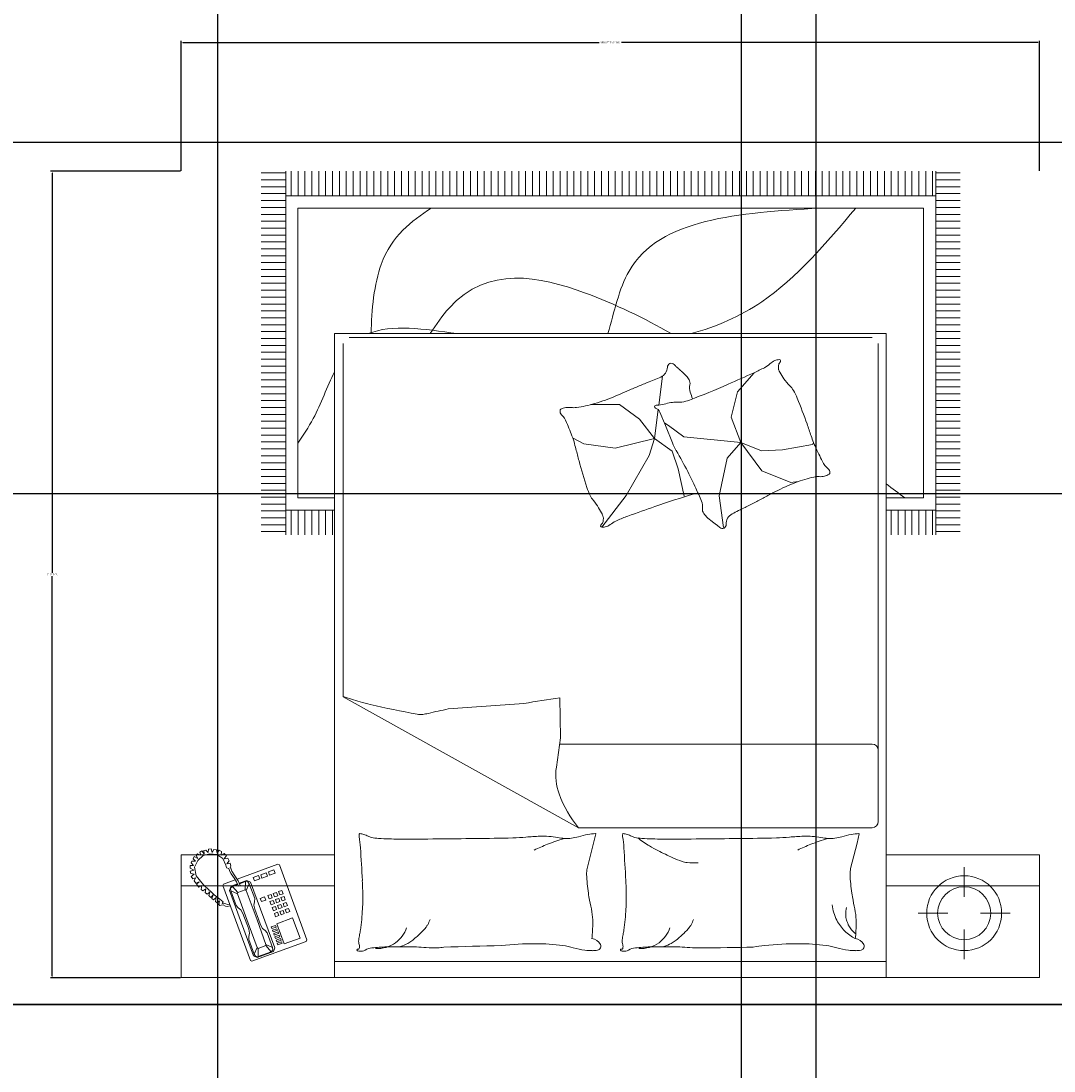
# Model space of a CAD drawing. Units: inches. Extents: x 318 to 927, y -1130 to 13.
# Tile 3 of 17: x 431 to 541, y -1041 to -929. Entities that reach past the tile are written whole.
import ezdxf

# ---------------------------------------------------------------- set-up
doc = ezdxf.new("R2010")
doc.units = ezdxf.units.IN
doc.header["$MEASUREMENT"] = 0
doc.layers.add('A-ANNO-DIMS', color=1, linetype='Continuous', lineweight=18)
doc.layers.add('wall', color=1, linetype='Continuous', lineweight=35)
doc.layers.add('furniture', color=50, linetype='Continuous', lineweight=13, transparency=0.8)
doc.styles.add('DIM_FONT', font='SIMPLEX.shx', dxfattribs={"width": 0.8})
doc.styles.get("Standard").update_dxf_attribs({"font": 'arial.ttf'})
doc.dimstyles.get("Standard").update_dxf_attribs({"dimtxt": 0.18, "dimasz": 0.18, "dimexe": 0.18, "dimexo": 0.0625, "dimgap": 0.09, "dimtad": 0, "dimtih": 1, "dimtoh": 1, "dimdec": 1, "dimzin": 0, "dimdsep": 46, "dimlunit": 4, "dimtxsty": 'Standard', "dimcen": 0.09, "dimadec": 0, "dimazin": 0, "dimtfac": 1, "dimtdec": 1, "dimtofl": 0, "dimtmove": 0, "dimatfit": 3, "dimfxl": 1, "dimtolj": 1, "dimtzin": 0, "dimarcsym": 0})

# ---------------------------------------------------------------- blocks, each defined once
blk = doc.blocks.new('A$C4F634EDD')
for p, q in [((0, 2.6295), (0, 2.2295)), ((0.5, 2.6295), (0, 2.6295)), ((0.5, 2.6295), (2.3, 2.6295)), ((0.5, 0.5295), (0.5, 2.6295)), ((0.5, 2.2295), (0.5, 2.6295)), ((2.3, 2.6295), (2.3, 0.5295)), ((2.3, 2.6295), (2.8, 2.6295)), ((2.3, 2.2295), (2.3, 2.6295)), ((2.8, 2.6295), (2.8, 2.2295)), ((0.2457, 2.5697), (0.2457, 2.4733)), ((0.5, 2.5771), (2.3, 2.5771)), ((2.392, 2.5115), (2.5692, 2.5765)), ((2.5692, 2.5765), (2.574, 2.5743)), ((2.574, 2.5743), (2.6638, 2.3298)), ((2.4946, 2.5331), (2.4985, 2.5445)), ((2.4985, 2.5445), (2.5516, 2.564)), ((2.5062, 2.5454), (2.5004, 2.5392)), ((2.5004, 2.5392), (2.5013, 2.5315)), ((2.5062, 2.5454), (2.5487, 2.561)), ((2.5235, 2.5256), (2.5062, 2.5454)), ((2.5483, 2.5347), (2.5235, 2.5256)), ((2.5483, 2.5347), (2.5487, 2.561)), ((2.5514, 2.5318), (2.5483, 2.5347)), ((2.5487, 2.561), (2.5571, 2.56)), ((2.5615, 2.5536), (2.5514, 2.5318)), ((2.5516, 2.564), (2.5637, 2.5584)), ((2.5571, 2.56), (2.5615, 2.5536)), ((2.5615, 2.5536), (2.5791, 2.5058)), ((2.5637, 2.5584), (2.6418, 2.3458)), ((2.3898, 2.5066), (2.392, 2.5115)), ((2.4795, 2.2621), (2.3898, 2.5066)), ((2.412, 2.5007), (2.4634, 2.5196)), ((2.4361, 2.4352), (2.412, 2.5007)), ((2.4634, 2.5196), (2.4875, 2.454)), ((2.4842, 2.5232), (2.47, 2.518)), ((2.47, 2.518), (2.472, 2.5127)), ((2.472, 2.5127), (2.4862, 2.5179)), ((2.4881, 2.5126), (2.4739, 2.5074)), ((2.4739, 2.5074), (2.4759, 2.502)), ((2.4759, 2.502), (2.4901, 2.5073)), ((2.492, 2.5019), (2.4778, 2.4967)), ((2.4862, 2.5179), (2.4842, 2.5232)), ((2.4901, 2.5073), (2.4881, 2.5126)), ((2.494, 2.4966), (2.492, 2.5019)), ((2.5734, 2.3187), (2.4946, 2.5331)), ((2.5013, 2.5315), (2.5188, 2.4836)), ((2.5013, 2.5315), (2.5231, 2.5214)), ((2.5231, 2.5214), (2.5235, 2.5256)), ((2.5523, 2.4417), (2.5231, 2.5214)), ((2.5807, 2.4521), (2.5514, 2.5318)), ((2.5791, 2.5058), (2.5788, 2.4956)), ((2.4778, 2.4967), (2.4798, 2.4914)), ((2.4798, 2.4914), (2.494, 2.4966)), ((2.4959, 2.4913), (2.4817, 2.4861)), ((2.4817, 2.4861), (2.4837, 2.4808)), ((2.4837, 2.4808), (2.4979, 2.486)), ((2.4998, 2.4807), (2.4856, 2.4755)), ((2.4856, 2.4755), (2.4876, 2.4702)), ((2.4876, 2.4702), (2.5018, 2.4754)), ((2.5037, 2.47), (2.4895, 2.4648)), ((2.4979, 2.486), (2.4959, 2.4913)), ((2.5018, 2.4754), (2.4998, 2.4807)), ((2.5057, 2.4647), (2.5037, 2.47)), ((2.5188, 2.4836), (2.5256, 2.4761)), ((2.5256, 2.4761), (2.5342, 2.4692)), ((2.5342, 2.4692), (2.5405, 2.4574)), ((2.5788, 2.4956), (2.5767, 2.4848)), ((2.5767, 2.4848), (2.5795, 2.4717)), ((2.5795, 2.4717), (2.586, 2.454)), ((2.4875, 2.454), (2.4361, 2.4352)), ((2.4895, 2.4648), (2.4915, 2.4595)), ((2.4915, 2.4595), (2.5057, 2.4647)), ((2.5405, 2.4574), (2.547, 2.4397)), ((2.5594, 2.4061), (2.547, 2.4397)), ((2.5523, 2.4417), (2.5875, 2.346)), ((2.5807, 2.4521), (2.6158, 2.3564)), ((2.5984, 2.4204), (2.586, 2.454)), ((0.0957, 2.4197), (0.192, 2.4197)), ((0.2994, 2.4197), (0.3957, 2.4197)), ((2.4457, 2.4146), (2.4563, 2.4185)), ((2.4496, 2.4039), (2.4457, 2.4146)), ((2.4602, 2.4078), (2.4496, 2.4039)), ((2.4528, 2.3951), (2.4635, 2.399)), ((2.4563, 2.4185), (2.4602, 2.4078)), ((2.4634, 2.4211), (2.474, 2.425)), ((2.4673, 2.4104), (2.4634, 2.4211)), ((2.4635, 2.399), (2.4674, 2.3883)), ((2.4779, 2.4143), (2.4673, 2.4104)), ((2.4706, 2.4016), (2.4812, 2.4055)), ((2.4745, 2.3909), (2.4706, 2.4016)), ((2.474, 2.425), (2.4779, 2.4143)), ((2.4811, 2.4276), (2.4917, 2.4315)), ((2.485, 2.4169), (2.4811, 2.4276)), ((2.4812, 2.4055), (2.4851, 2.3949)), ((2.4956, 2.4208), (2.485, 2.4169)), ((2.4883, 2.4081), (2.4989, 2.412)), ((2.4922, 2.3975), (2.4883, 2.4081)), ((2.4917, 2.4315), (2.4956, 2.4208)), ((2.5028, 2.4014), (2.4922, 2.3975)), ((2.4989, 2.412), (2.5028, 2.4014)), ((2.5622, 2.393), (2.5594, 2.4061)), ((2.6047, 2.4086), (2.5984, 2.4204)), ((2.6133, 2.4017), (2.6047, 2.4086)), ((2.6201, 2.3941), (2.6133, 2.4017)), ((2.6499, 2.3979), (2.6397, 2.3953)), ((2.6551, 2.397), (2.6499, 2.3979)), ((0.2457, 2.366), (0.2457, 2.2697)), ((2.4567, 2.3844), (2.4528, 2.3951)), ((2.4674, 2.3883), (2.4567, 2.3844)), ((2.46, 2.3756), (2.4706, 2.3795)), ((2.4639, 2.365), (2.46, 2.3756)), ((2.4745, 2.3689), (2.4639, 2.365)), ((2.4706, 2.3795), (2.4745, 2.3689)), ((2.4851, 2.3949), (2.4745, 2.3909)), ((2.4777, 2.3821), (2.4883, 2.386)), ((2.4816, 2.3715), (2.4777, 2.3821)), ((2.4922, 2.3754), (2.4816, 2.3715)), ((2.4849, 2.3626), (2.4955, 2.3665)), ((2.4883, 2.386), (2.4922, 2.3754)), ((2.4954, 2.3886), (2.5061, 2.3925)), ((2.4993, 2.378), (2.4954, 2.3886)), ((2.4955, 2.3665), (2.4994, 2.3559)), ((2.51, 2.3819), (2.4993, 2.378)), ((2.5026, 2.3691), (2.5132, 2.373)), ((2.5065, 2.3585), (2.5026, 2.3691)), ((2.5061, 2.3925), (2.51, 2.3819)), ((2.5132, 2.373), (2.5171, 2.3624)), ((2.5238, 2.3769), (2.538, 2.3821)), ((2.5277, 2.3663), (2.5238, 2.3769)), ((2.5419, 2.3715), (2.5277, 2.3663)), ((2.538, 2.3821), (2.5419, 2.3715)), ((2.5598, 2.372), (2.5601, 2.3822)), ((2.5774, 2.3242), (2.5598, 2.372)), ((2.5601, 2.3822), (2.5622, 2.393)), ((2.6376, 2.3463), (2.6201, 2.3941)), ((2.6417, 2.39), (2.6488, 2.391)), ((2.6488, 2.391), (2.6538, 2.3895)), ((2.6538, 2.3895), (2.6596, 2.388)), ((2.6627, 2.392), (2.6551, 2.397)), ((2.6596, 2.388), (2.6626, 2.3867)), ((2.6626, 2.3867), (2.6662, 2.388)), ((2.6692, 2.394), (2.6627, 2.392)), ((2.6662, 2.388), (2.6632, 2.3828)), ((2.6632, 2.3828), (2.6736, 2.3744)), ((2.6736, 2.3944), (2.6692, 2.394)), ((2.6765, 2.391), (2.6736, 2.3944)), ((2.6736, 2.3744), (2.6922, 2.3593)), ((2.6742, 2.3795), (2.6765, 2.391)), ((2.6824, 2.3858), (2.6742, 2.3795)), ((2.6873, 2.3815), (2.6824, 2.3858)), ((2.6853, 2.369), (2.6873, 2.3815)), ((2.6946, 2.376), (2.6853, 2.369)), ((2.6995, 2.3713), (2.6946, 2.376)), ((2.695, 2.3603), (2.6995, 2.3713)), ((2.7031, 2.3682), (2.695, 2.3603)), ((2.7096, 2.3616), (2.7031, 2.3682)), ((0, 2.3301), (0.5, 2.3301)), ((2.8, 2.3301), (2.3, 2.3301)), ((2.4672, 2.3561), (2.4778, 2.36)), ((2.4711, 2.3455), (2.4672, 2.3561)), ((2.4817, 2.3494), (2.4711, 2.3455)), ((2.4778, 2.36), (2.4817, 2.3494)), ((2.4888, 2.352), (2.4849, 2.3626)), ((2.4994, 2.3559), (2.4888, 2.352)), ((2.5171, 2.3624), (2.5065, 2.3585)), ((2.5774, 2.3242), (2.5875, 2.346)), ((2.5875, 2.346), (2.5905, 2.3431)), ((2.5905, 2.3431), (2.5901, 2.3168)), ((2.6154, 2.3522), (2.5905, 2.3431)), ((2.613, 2.3312), (2.6077, 2.3293)), ((2.6077, 2.3293), (2.6135, 2.3141)), ((2.6192, 2.3174), (2.613, 2.3312)), ((2.6153, 2.3261), (2.6327, 2.3324)), ((2.6158, 2.3564), (2.6154, 2.3522)), ((2.6154, 2.3522), (2.6327, 2.3324)), ((2.6376, 2.3463), (2.6158, 2.3564)), ((2.6369, 2.332), (2.6161, 2.3243)), ((2.6327, 2.3324), (2.6385, 2.3386)), ((2.6418, 2.3458), (2.6369, 2.332)), ((2.6385, 2.3386), (2.6376, 2.3463)), ((2.6638, 2.3298), (2.6616, 2.3249)), ((2.6922, 2.3593), (2.7051, 2.3473)), ((2.7051, 2.3473), (2.7079, 2.3475)), ((2.7062, 2.351), (2.7096, 2.3616)), ((2.7147, 2.3578), (2.7062, 2.351)), ((2.7079, 2.3475), (2.7079, 2.3443)), ((2.7079, 2.3443), (2.727, 2.3277)), ((2.7214, 2.3517), (2.7147, 2.3578)), ((2.7196, 2.34), (2.7214, 2.3517)), ((2.7286, 2.3466), (2.7196, 2.34)), ((2.7346, 2.3423), (2.7286, 2.3466)), ((2.732, 2.3295), (2.7346, 2.3423)), ((2.7423, 2.3345), (2.732, 2.3295)), ((2.7495, 2.325), (2.7423, 2.3345)), ((2.6172, 2.3086), (2.4844, 2.2599)), ((2.5114, 2.2959), (2.4936, 2.2894)), ((2.5153, 2.2853), (2.5114, 2.2959)), ((2.5362, 2.305), (2.5185, 2.2985)), ((2.5185, 2.2985), (2.5224, 2.2879)), ((2.5401, 2.2944), (2.5362, 2.305)), ((2.561, 2.3141), (2.5433, 2.3076)), ((2.5433, 2.3076), (2.5472, 2.297)), ((2.5472, 2.297), (2.5649, 2.3035)), ((2.5649, 2.3035), (2.561, 2.3141)), ((2.5855, 2.3131), (2.5734, 2.3187)), ((2.5818, 2.3178), (2.5774, 2.3242)), ((2.5901, 2.3168), (2.5818, 2.3178)), ((2.6104, 2.3222), (2.5855, 2.3131)), ((2.5901, 2.3168), (2.6097, 2.324)), ((2.6135, 2.3141), (2.6244, 2.2977)), ((2.626, 2.3069), (2.6192, 2.3174)), ((2.6616, 2.3249), (2.6234, 2.3109)), ((2.6244, 2.2977), (2.6349, 2.2825)), ((2.6365, 2.2916), (2.626, 2.3069)), ((2.727, 2.3277), (2.7512, 2.2983)), ((2.7406, 2.3172), (2.7495, 2.325)), ((2.7519, 2.3218), (2.7406, 2.3172)), ((2.7512, 2.2983), (2.756, 2.2695)), ((2.7575, 2.3144), (2.7519, 2.3218)), ((2.7526, 2.3045), (2.7575, 2.3144)), ((2.7622, 2.308), (2.7526, 2.3045)), ((2.7574, 2.2924), (2.7673, 2.2997)), ((2.7673, 2.2997), (2.7622, 2.308)), ((0.5953, 2.1912), (0.616, 2.2738)), ((1.4546, 2.1912), (1.4752, 2.2738)), ((2.4844, 2.2599), (2.4795, 2.2621)), ((2.4936, 2.2894), (2.4976, 2.2788)), ((2.4976, 2.2788), (2.5153, 2.2853)), ((2.5224, 2.2879), (2.5401, 2.2944)), ((2.6349, 2.2825), (2.638, 2.273)), ((2.6407, 2.2834), (2.6365, 2.2916)), ((2.6399, 2.2712), (2.6374, 2.2659)), ((2.6374, 2.2659), (2.6398, 2.257)), ((2.638, 2.273), (2.6399, 2.2712)), ((2.6438, 2.2739), (2.6407, 2.2834)), ((2.6519, 2.2716), (2.6438, 2.2739)), ((2.6535, 2.2628), (2.6519, 2.2716)), ((2.6636, 2.2409), (2.6535, 2.2628)), ((2.756, 2.2695), (2.7459, 2.2483)), ((2.7687, 2.2905), (2.7574, 2.2924)), ((2.7587, 2.279), (2.7699, 2.2828)), ((2.7708, 2.2725), (2.7587, 2.279)), ((2.759, 2.2637), (2.7706, 2.2643)), ((2.7676, 2.2559), (2.759, 2.2637)), ((2.7699, 2.2828), (2.7687, 2.2905)), ((2.7706, 2.2643), (2.7708, 2.2725)), ((0, 2.2295), (0.5, 2.2295)), ((2.8, 2.2295), (2.3, 2.2295)), ((2.6398, 2.257), (2.6509, 2.259)), ((2.6509, 2.259), (2.6431, 2.2492)), ((2.6431, 2.2492), (2.6473, 2.2398)), ((2.6473, 2.2398), (2.6592, 2.2429)), ((2.6592, 2.2429), (2.6521, 2.2314)), ((2.6521, 2.2314), (2.6598, 2.2248)), ((2.6598, 2.2248), (2.6697, 2.2309)), ((2.6836, 2.2287), (2.6636, 2.2409)), ((2.6697, 2.2309), (2.6684, 2.219)), ((2.7063, 2.2256), (2.6836, 2.2287)), ((2.7284, 2.2317), (2.7063, 2.2256)), ((2.7255, 2.2152), (2.7242, 2.2265)), ((2.7242, 2.2265), (2.7324, 2.2165)), ((2.7459, 2.2483), (2.7284, 2.2317)), ((2.7386, 2.2208), (2.7354, 2.2306)), ((2.7354, 2.2306), (2.7462, 2.2264)), ((2.7509, 2.2314), (2.7459, 2.2418)), ((2.7459, 2.2418), (2.7568, 2.2352)), ((2.7462, 2.2264), (2.7509, 2.2314)), ((2.7529, 2.2505), (2.7645, 2.2498)), ((2.7607, 2.2424), (2.7529, 2.2505)), ((2.7568, 2.2352), (2.7607, 2.2424)), ((2.7645, 2.2498), (2.7676, 2.2559)), ((2.6684, 2.219), (2.6761, 2.2145)), ((2.6761, 2.2145), (2.6821, 2.2237)), ((2.6821, 2.2237), (2.6843, 2.2135)), ((2.6843, 2.2135), (2.6927, 2.2117)), ((2.6927, 2.2117), (2.6986, 2.222)), ((2.6986, 2.222), (2.7019, 2.2098)), ((2.7019, 2.2098), (2.7102, 2.2104)), ((2.7102, 2.2104), (2.7113, 2.2218)), ((2.7113, 2.2218), (2.7192, 2.2137)), ((2.7192, 2.2137), (2.7255, 2.2152)), ((2.7324, 2.2165), (2.7386, 2.2208)), ((0.5878, 2.1612), (0.5953, 2.1912)), ((1.4471, 2.1612), (1.4546, 2.1912)), ((1.5035, 2.141), (0.5458, 2.141)), ((1.5035, 2.141), (2.2716, 1.7136)), ((0.5258, 2.121), (0.5258, 0.5617)), ((1.576, 1.9433), (1.5624, 1.8479)), ((0.5458, 1.8684), (1.5653, 1.8684)), ((1.5624, 1.8479), (1.5641, 1.7178)), ((2.2716, 0.5617), (2.2716, 1.7136)), ((0.2586, 1.1753), (0.3386, 1.1753)), ((0.3386, 0), (0.3386, 1.1852)), ((0.3486, 1.1052), (0.3486, 1.1852)), ((0.3711, 1.1052), (0.3711, 1.1852)), ((0.3936, 1.1052), (0.3936, 1.1852)), ((0.4161, 1.1052), (0.4161, 1.1852)), ((0.4386, 1.1052), (0.4386, 1.1852)), ((0.4611, 1.1052), (0.4611, 1.1852)), ((0.4836, 1.1052), (0.4836, 1.1852)), ((2.3061, 1.1052), (2.3061, 1.1852)), ((2.3286, 1.1052), (2.3286, 1.1852)), ((2.3511, 1.1052), (2.3511, 1.1852)), ((2.3736, 1.1052), (2.3736, 1.1852)), ((2.3961, 1.1052), (2.3961, 1.1852)), ((2.4186, 1.1052), (2.4186, 1.1852)), ((2.4411, 1.1052), (2.4411, 1.1852)), ((2.4588, 1.1852), (2.4588, 0)), ((2.4588, 1.1753), (2.5388, 1.1753)), ((0.2586, 1.1528), (0.3386, 1.1528)), ((0.2586, 1.1303), (0.3386, 1.1303)), ((1.031, 1.1612), (1.0448, 1.0581)), ((1.4276, 1.1611), (1.3484, 1.0571)), ((2.4588, 1.1528), (2.5388, 1.1528)), ((2.4588, 1.1303), (2.5388, 1.1303)), ((0.2586, 1.1078), (0.3386, 1.1078)), ((0.3386, 1.1052), (0.5, 1.1052)), ((2.3, 1.1052), (2.4588, 1.1052)), ((2.4588, 1.1078), (2.5388, 1.1078)), ((0.2586, 1.0853), (0.3386, 1.0853)), ((0.2586, 1.0628), (0.3386, 1.0628)), ((0.3786, 1.0652), (0.5, 1.0652)), ((0.3786, 0.12), (0.3786, 1.0652)), ((2.3, 1.0652), (2.4188, 1.0652)), ((2.4188, 1.0652), (2.4188, 0.12)), ((2.4588, 1.0853), (2.5388, 1.0853)), ((2.4588, 1.0628), (2.5388, 1.0628)), ((0.2586, 1.0403), (0.3386, 1.0403)), ((1.0448, 1.0581), (1.019, 0.936)), ((1.1784, 0.9702), (1.1586, 1.0591)), ((1.3484, 1.0571), (1.2733, 0.9268)), ((2.4588, 1.0403), (2.5388, 1.0403)), ((0.2586, 1.0178), (0.3386, 1.0178)), ((0.2586, 0.9953), (0.3386, 0.9953)), ((0.8108, 1.0151), (0.7868, 1.0117)), ((0.9054, 0.9773), (0.8108, 1.0151)), ((2.4588, 1.0178), (2.5388, 1.0178)), ((2.4588, 0.9953), (2.5388, 0.9953)), ((0.2586, 0.9728), (0.3386, 0.9728)), ((0.9743, 0.8845), (0.9054, 0.9773)), ((1.1982, 0.9129), (1.1784, 0.9702)), ((2.4588, 0.9728), (2.5388, 0.9728)), ((0.2586, 0.9503), (0.3386, 0.9503)), ((0.2586, 0.9278), (0.3386, 0.9278)), ((1.019, 0.936), (0.9743, 0.8845)), ((1.2733, 0.9268), (1.2555, 0.8715)), ((2.4588, 0.9503), (2.5388, 0.9503)), ((2.4588, 0.9278), (2.5388, 0.9278)), ((0.2586, 0.9053), (0.3386, 0.9053)), ((0.7403, 0.8913), (0.737, 0.8849)), ((0.8384, 0.9085), (0.7403, 0.8913)), ((0.9072, 0.912), (0.8384, 0.9085)), ((0.9743, 0.8845), (0.9072, 0.912)), ((1.2555, 0.8715), (1.1982, 0.9129)), ((1.2555, 0.8715), (1.384, 0.9031)), ((1.384, 0.9031), (1.4868, 0.8892)), ((2.4588, 0.9053), (2.5388, 0.9053)), ((0.2586, 0.8828), (0.3386, 0.8828)), ((0.2586, 0.8603), (0.3386, 0.8603)), ((0.9743, 0.8845), (1.0052, 0.802)), ((0.9743, 0.8845), (1.16, 0.8656)), ((1.16, 0.8656), (1.2099, 0.8295)), ((1.1973, 0.8853), (1.2203, 0.829)), ((1.2555, 0.8715), (1.2437, 0.7773)), ((1.2555, 0.8715), (1.3049, 0.8082)), ((1.4868, 0.8892), (1.5228, 0.8692)), ((2.4588, 0.8828), (2.5388, 0.8828)), ((2.4588, 0.8603), (2.5388, 0.8603)), ((0.2586, 0.8378), (0.3386, 0.8378)), ((1.2099, 0.8295), (1.222, 0.8209)), ((1.2203, 0.829), (1.2381, 0.7855)), ((2.4588, 0.8378), (2.5388, 0.8378)), ((0.2586, 0.8153), (0.3386, 0.8153)), ((0.2586, 0.7928), (0.3386, 0.7928)), ((1.0052, 0.802), (0.9846, 0.7194)), ((1.3049, 0.8082), (1.3701, 0.7608)), ((2.4588, 0.8153), (2.5388, 0.8153)), ((2.4588, 0.7928), (2.5388, 0.7928)), ((0.2586, 0.7703), (0.3386, 0.7703)), ((1.2419, 0.7626), (1.23, 0.668)), ((1.3701, 0.7608), (1.463, 0.7608)), ((2.4588, 0.7703), (2.5388, 0.7703)), ((0.2586, 0.7478), (0.3386, 0.7478)), ((0.2586, 0.7253), (0.3386, 0.7253)), ((0.9846, 0.7194), (0.931, 0.6569)), ((2.4588, 0.7478), (2.5388, 0.7478)), ((2.4588, 0.7253), (2.5388, 0.7253)), ((0.2586, 0.7028), (0.3386, 0.7028)), ((2.4588, 0.7028), (2.5388, 0.7028)), ((0.2586, 0.6803), (0.3386, 0.6803)), ((0.2586, 0.6578), (0.3386, 0.6578)), ((2.4588, 0.6803), (2.5388, 0.6803)), ((2.4588, 0.6578), (2.5388, 0.6578)), ((0.2586, 0.6353), (0.3386, 0.6353)), ((2.4588, 0.6353), (2.5388, 0.6353)), ((0.2586, 0.6128), (0.3386, 0.6128)), ((0.2586, 0.5903), (0.3386, 0.5903)), ((2.4588, 0.6128), (2.5388, 0.6128)), ((2.4588, 0.5903), (2.5388, 0.5903)), ((0.2586, 0.5678), (0.3386, 0.5678)), ((2.4588, 0.5678), (2.5388, 0.5678)), ((0.2586, 0.5453), (0.3386, 0.5453)), ((0.2586, 0.5228), (0.3386, 0.5228)), ((2.3, 0.5295), (0.5, 0.5295)), ((0.5458, 0.5417), (2.2516, 0.5417)), ((2.4588, 0.5453), (2.5388, 0.5453)), ((2.4588, 0.5228), (2.5388, 0.5228)), ((0.2586, 0.5003), (0.3386, 0.5003)), ((2.4588, 0.5003), (2.5388, 0.5003)), ((0.2586, 0.4778), (0.3386, 0.4778)), ((0.2586, 0.4553), (0.3386, 0.4553)), ((2.4588, 0.4778), (2.5388, 0.4778)), ((2.4588, 0.4553), (2.5388, 0.4553)), ((0.2586, 0.4328), (0.3386, 0.4328)), ((2.4588, 0.4328), (2.5388, 0.4328)), ((0.2586, 0.4103), (0.3386, 0.4103)), ((0.2586, 0.3878), (0.3386, 0.3878)), ((2.4588, 0.4103), (2.5388, 0.4103)), ((2.4588, 0.3878), (2.5388, 0.3878)), ((0.2586, 0.3653), (0.3386, 0.3653)), ((0.2586, 0.3428), (0.3386, 0.3428)), ((2.4588, 0.3653), (2.5388, 0.3653)), ((2.4588, 0.3428), (2.5388, 0.3428)), ((0.2586, 0.3203), (0.3386, 0.3203)), ((2.4588, 0.3203), (2.5388, 0.3203)), ((0.2586, 0.2978), (0.3386, 0.2978)), ((0.2586, 0.2753), (0.3386, 0.2753)), ((2.4588, 0.2978), (2.5388, 0.2978)), ((2.4588, 0.2753), (2.5388, 0.2753)), ((0.2586, 0.2528), (0.3386, 0.2528)), ((2.4588, 0.2528), (2.5388, 0.2528)), ((0.2586, 0.2303), (0.3386, 0.2303)), ((0.2586, 0.2078), (0.3386, 0.2078)), ((2.4588, 0.2303), (2.5388, 0.2303)), ((2.4588, 0.2078), (2.5388, 0.2078)), ((0.2586, 0.1853), (0.3386, 0.1853)), ((2.4588, 0.1853), (2.5388, 0.1853)), ((0.2586, 0.1628), (0.3386, 0.1628)), ((0.2586, 0.1403), (0.3386, 0.1403)), ((2.4588, 0.1628), (2.5388, 0.1628)), ((2.4588, 0.1403), (2.5388, 0.1403)), ((0.2586, 0.1178), (0.3386, 0.1178)), ((2.4188, 0.12), (0.3786, 0.12)), ((2.4588, 0.1178), (2.5388, 0.1178)), ((0.2586, 0.0953), (0.3386, 0.0953)), ((0.2586, 0.0728), (0.3386, 0.0728)), ((2.4588, 0.08), (0.3386, 0.08)), ((0.3486, 0), (0.3486, 0.08)), ((0.3711, 0), (0.3711, 0.08)), ((0.3936, 0), (0.3936, 0.08)), ((0.4161, 0), (0.4161, 0.08)), ((0.4386, 0), (0.4386, 0.08)), ((0.4611, 0), (0.4611, 0.08)), ((0.4836, 0), (0.4836, 0.08)), ((0.5061, 0), (0.5061, 0.08)), ((0.5286, 0), (0.5286, 0.08)), ((0.5511, 0), (0.5511, 0.08)), ((0.5736, 0), (0.5736, 0.08)), ((0.5961, 0), (0.5961, 0.08)), ((0.6186, 0), (0.6186, 0.08)), ((0.6411, 0), (0.6411, 0.08)), ((0.6636, 0), (0.6636, 0.08)), ((0.6861, 0), (0.6861, 0.08)), ((0.7086, 0), (0.7086, 0.08)), ((0.7311, 0), (0.7311, 0.08)), ((0.7536, 0), (0.7536, 0.08)), ((0.7761, 0), (0.7761, 0.08)), ((0.7986, 0), (0.7986, 0.08)), ((0.8211, 0), (0.8211, 0.08)), ((0.8436, 0), (0.8436, 0.08)), ((0.8661, 0), (0.8661, 0.08)), ((0.8886, 0), (0.8886, 0.08)), ((0.9111, 0), (0.9111, 0.08)), ((0.9336, 0), (0.9336, 0.08)), ((0.9561, 0), (0.9561, 0.08)), ((0.9786, 0), (0.9786, 0.08)), ((1.0011, 0), (1.0011, 0.08)), ((1.0236, 0), (1.0236, 0.08)), ((1.0461, 0), (1.0461, 0.08)), ((1.0686, 0), (1.0686, 0.08)), ((1.0911, 0), (1.0911, 0.08)), ((1.1136, 0), (1.1136, 0.08)), ((1.1361, 0), (1.1361, 0.08)), ((1.1586, 0), (1.1586, 0.08)), ((1.1811, 0), (1.1811, 0.08)), ((1.2036, 0), (1.2036, 0.08)), ((1.2261, 0), (1.2261, 0.08)), ((1.2486, 0), (1.2486, 0.08)), ((1.2711, 0), (1.2711, 0.08)), ((1.2936, 0), (1.2936, 0.08)), ((1.3161, 0), (1.3161, 0.08)), ((1.3386, 0), (1.3386, 0.08)), ((1.3611, 0), (1.3611, 0.08)), ((1.3836, 0), (1.3836, 0.08)), ((1.4061, 0), (1.4061, 0.08)), ((1.4286, 0), (1.4286, 0.08)), ((1.4511, 0), (1.4511, 0.08)), ((1.4736, 0), (1.4736, 0.08)), ((1.4961, 0), (1.4961, 0.08)), ((1.5186, 0), (1.5186, 0.08)), ((1.5411, 0), (1.5411, 0.08)), ((1.5636, 0), (1.5636, 0.08)), ((1.5861, 0), (1.5861, 0.08)), ((1.6086, 0), (1.6086, 0.08)), ((1.6311, 0), (1.6311, 0.08)), ((1.6536, 0), (1.6536, 0.08)), ((1.6761, 0), (1.6761, 0.08)), ((1.6986, 0), (1.6986, 0.08)), ((1.7211, 0), (1.7211, 0.08)), ((1.7436, 0), (1.7436, 0.08)), ((1.7661, 0), (1.7661, 0.08)), ((1.7886, 0), (1.7886, 0.08)), ((1.8111, 0), (1.8111, 0.08)), ((1.8336, 0), (1.8336, 0.08)), ((1.8561, 0), (1.8561, 0.08)), ((1.8786, 0), (1.8786, 0.08)), ((1.9011, 0), (1.9011, 0.08)), ((1.9236, 0), (1.9236, 0.08)), ((1.9461, 0), (1.9461, 0.08)), ((1.9686, 0), (1.9686, 0.08)), ((1.9911, 0), (1.9911, 0.08)), ((2.0136, 0), (2.0136, 0.08)), ((2.0361, 0), (2.0361, 0.08)), ((2.0586, 0), (2.0586, 0.08)), ((2.0811, 0), (2.0811, 0.08)), ((2.1036, 0), (2.1036, 0.08)), ((2.1261, 0), (2.1261, 0.08)), ((2.1486, 0), (2.1486, 0.08)), ((2.1711, 0), (2.1711, 0.08)), ((2.1936, 0), (2.1936, 0.08)), ((2.2161, 0), (2.2161, 0.08)), ((2.2386, 0), (2.2386, 0.08)), ((2.2611, 0), (2.2611, 0.08)), ((2.2836, 0), (2.2836, 0.08)), ((2.3061, 0), (2.3061, 0.08)), ((2.3286, 0), (2.3286, 0.08)), ((2.3511, 0), (2.3511, 0.08)), ((2.3736, 0), (2.3736, 0.08)), ((2.3961, 0), (2.3961, 0.08)), ((2.4186, 0), (2.4186, 0.08)), ((2.4411, 0), (2.4411, 0.08)), ((2.4588, 0.0953), (2.5388, 0.0953)), ((2.4588, 0.0728), (2.5388, 0.0728)), ((0.2586, 0.0503), (0.3386, 0.0503)), ((2.4588, 0.0503), (2.5388, 0.0503)), ((0.2586, 0.0278), (0.3386, 0.0278)), ((0.2586, 0.0053), (0.3386, 0.0053)), ((2.4588, 0.0278), (2.5388, 0.0278)), ((2.4588, 0.0053), (2.5388, 0.0053))]:
    blk.add_line(p, q)
for radius in [0.1222, 0.0865]:
    blk.add_circle((0.2457, 2.4197), radius)
for centre, radius, start, end in [((0.5848, 2.5274), 0.0131, 101.2724, 206.5805), ((0.5999, 2.4516), 0.0904, 90, 101.2724), ((0.5999, 2.3808), 0.1611, 81.5628, 90), ((0.5788, 2.2388), 0.3048, 74.256, 81.5628), ((1.2995, 2.4357), 0.0992, 85.7841, 105.9352), ((1.3132, 2.5864), 0.0539, 275.2592, 300.6513), ((1.3554, 2.5152), 0.0289, 85.6975, 120.6513), ((1.3556, 2.519), 0.0251, 68.2117, 85.6975), ((1.3739, 2.5288), 0.0156, 158.0096, 201.421), ((1.3634, 2.533), 0.00428, 78.1069, 158.0096), ((1.3647, 2.5395), 0.00232, 258.1069, 19.564), ((1.3637, 2.5391), 0.00342, 19.564, 68.2117), ((1.444, 2.5274), 0.0131, 101.2724, 206.5805), ((1.4591, 2.4516), 0.0904, 90, 101.2724), ((1.4591, 2.3808), 0.1611, 81.5628, 90), ((1.438, 2.2388), 0.3048, 74.256, 81.5628), ((2.1588, 2.4357), 0.0992, 85.7841, 105.9352), ((2.1724, 2.5864), 0.0539, 275.2592, 300.6513), ((2.2146, 2.5152), 0.0289, 85.6975, 120.6513), ((2.2149, 2.519), 0.0251, 68.2117, 85.6975), ((2.2331, 2.5288), 0.0156, 158.0096, 201.421), ((2.2226, 2.533), 0.00428, 78.1069, 158.0096), ((2.224, 2.5395), 0.00232, 258.1069, 19.564), ((2.2229, 2.5391), 0.00342, 19.564, 68.2117), ((0.6036, 2.5368), 0.0342, 206.5805, 265.5998), ((1.0898, 2.4496), 0.4918, 173.7676, 180), ((0.5368, 2.3783), 0.1399, 45.0976, 62.7964), ((0.7272, 2.7653), 0.2422, 254.256, 262.4531), ((0.7851, 3.2019), 0.6827, 262.4531, 270), ((0.7851, 3.5682), 1.049, 270, 276.0867), ((0.8402, 3.0514), 0.5293, 276.0867, 280.1899), ((1.1602, -8.1346), 10.6675, 90.30153, 91.21582), ((1.1169, 2.2433), 0.2897, 85.1982, 92.5386), ((1.2142, 3.4021), 0.8732, 265.1982, 269.4243), ((1.4317, 2.2032), 0.3916, 128.3886, 133.8115), ((1.2362, 2.45), 0.0768, 117.2396, 128.3886), ((1.3082, 2.3102), 0.234, 110.8603, 117.2396), ((1.2204, 4.0232), 1.4943, 269.4243, 271.9079), ((1.2995, 2.4357), 0.0992, 126.0864, 143.8234), ((1.2995, 2.4357), 0.0992, 105.9352, 126.0864), ((1.2429, 3.3501), 0.8208, 271.9079, 275.2592), ((1.1177, 2.5413), 0.246, 347.8905, 351.8665), ((1.3288, 2.5111), 0.0328, 351.8665, 21.421), ((1.4628, 2.5368), 0.0342, 206.5805, 265.5998), ((1.949, 2.4496), 0.4918, 173.7676, 180), ((1.5865, 2.7653), 0.2422, 254.256, 262.4531), ((1.6443, 3.2019), 0.6827, 262.4531, 270), ((1.6443, 3.5682), 1.049, 270, 276.0867), ((1.4785, 15.4878), 12.9656, 271.22425, 272.05324), ((1.97, 2.3805), 0.1524, 92.5386, 100.1899), ((1.9761, 2.2433), 0.2897, 85.1982, 92.5386), ((2.0734, 3.4021), 0.8732, 265.1982, 269.4243), ((2.291, 2.2032), 0.3916, 128.3886, 133.8115), ((2.0954, 2.45), 0.0768, 117.2396, 128.3886), ((2.1674, 2.3102), 0.234, 110.8603, 117.2396), ((2.0797, 4.0232), 1.4943, 269.4243, 271.9079), ((2.1588, 2.4357), 0.0992, 126.0864, 143.8234), ((2.1588, 2.4357), 0.0992, 105.9352, 126.0864), ((2.1021, 3.3501), 0.8208, 271.9079, 275.2592), ((1.977, 2.5413), 0.246, 347.8905, 351.8665), ((2.1881, 2.5111), 0.0328, 351.8665, 21.421), ((0.5462, 2.4142), 0.0899, 41.4429, 53.7359), ((0.5741, 2.4389), 0.0526, 25.3551, 41.4429), ((0.5368, 2.3783), 0.1399, 27.3988, 45.0976), ((1.3165, 2.3233), 0.2252, 133.8115, 140.9651), ((1.2995, 2.4357), 0.0992, 143.8234, 161.5603), ((2.2605, 2.3525), 0.9131, 172.3191, 176.6313), ((1.5522, 2.448), 0.1983, 167.8905, 172.3191), ((2.1757, 2.3233), 0.2252, 133.8115, 140.9651), ((2.1588, 2.4357), 0.0992, 143.8234, 161.5603), ((3.1198, 2.3525), 0.9131, 172.3191, 176.6313), ((2.4114, 2.448), 0.1983, 167.8905, 172.3191), ((0.8019, 2.4496), 0.204, 180, 189.6844), ((0.4851, 2.3967), 0.1511, 21.8149, 25.3551), ((0.4345, 2.3765), 0.2056, 18.7799, 21.8149), ((0.576, 2.4246), 0.0562, 0, 18.7799), ((0.5368, 2.3783), 0.1399, 16.515, 27.3988), ((1.3127, 2.3625), 0.2002, 151.6832, 156.9972), ((1.1799, 2.4341), 0.0493, 140.9651, 151.6832), ((1.6611, 2.4496), 0.204, 180, 189.6844), ((2.1719, 2.3625), 0.2002, 151.6832, 156.9972), ((2.0391, 2.4341), 0.0493, 140.9651, 151.6832), ((1.4703, 2.5637), 0.882, 189.6844, 192.1984), ((0.5406, 2.4246), 0.0915, 345.3149, 0), ((0.5368, 2.3783), 0.1399, 5.6311, 16.515), ((2.0266, 2.3663), 0.6787, 176.6313, 181.6331), ((2.3295, 2.5637), 0.882, 189.6844, 192.1984), ((2.8858, 2.3663), 0.6787, 176.6313, 181.6331), ((0.2982, 2.3103), 0.3171, 8.0051, 12.1984), ((1.1575, 2.3103), 0.3171, 8.0051, 12.1984), ((-0.0401, 2.2627), 0.6588, 2.6649, 8.0051), ((2.7128, 2.3859), 1.3652, 181.6331, 183.055), ((0.8191, 2.2627), 0.6588, 2.6649, 8.0051), ((3.5721, 2.3859), 1.3652, 181.6331, 183.055), ((14.9657, 3.0398), 13.6356, 183.05496, 183.50486), ((15.8249, 3.0398), 13.6356, 183.05496, 183.50486), ((0.5503, 2.2902), 0.0677, 345.9548, 2.6649), ((1.4096, 2.2902), 0.0677, 345.9548, 2.6649), ((1.1303, 1.9835), 0.2721, 85.9172, 93.5552), ((1.1455, 2.197), 0.058, 69.3257, 85.9172), ((0.9871, 1.7772), 0.5066, 65.6735, 69.3257), ((0.6058, 0.9338), 1.4323, 63.5015, 65.6735), ((0.473, 2.8815), 0.7387, 289.428, 291.6577), ((0.473, 2.8815), 0.7387, 291.6577, 293.4844), ((0.473, 2.8815), 0.7387, 293.4844, 295.3111), ((1.1054, 1.9358), 0.3126, 57.865, 63.5015), ((0.8841, 1.5835), 0.7286, 54.1737, 57.865), ((1.6762, 2.2258), 0.3212, 183.5049, 189.9984), ((1.3322, 2.8815), 0.7387, 289.428, 291.6577), ((1.3322, 2.8815), 0.7387, 291.6577, 293.4844), ((1.3322, 2.8815), 0.7387, 293.4844, 295.3111), ((2.5355, 2.2258), 0.3212, 183.5049, 189.9984), ((0.5887, 2.1609), 0.000917, 165.9551, 274.0829), ((0.5695, 2.4301), 0.2708, 274.0829, 279.4841), ((0.5763, 2.3896), 0.2297, 279.4841, 287.3864), ((0.6807, 2.0561), 0.1197, 96.4341, 107.3864), ((0.6836, 2.0301), 0.1459, 78.4414, 96.4341), ((0.473, 2.8815), 0.7387, 287.1982, 289.428), ((0.759, 2.3985), 0.2301, 258.4414, 272.7491), ((0.7026, 3.5718), 1.4048, 272.7491, 274.6176), ((0.9136, 0.9591), 1.2165, 92.6096, 94.6176), ((1.2501, -19.8405), 22.0183, 90.37908, 91.01965), ((1.2012, -3.5404), 5.7185, 89.7135, 90.9704), ((1.224, 1.0141), 1.164, 86.426, 89.7135), ((1.2875, 2.0302), 0.1459, 77.131, 86.426), ((1.3099, 2.1283), 0.0453, 62.7159, 77.131), ((1.3658, 2.2367), 0.0767, 242.7159, 253.7788), ((1.3688, 2.247), 0.0875, 253.7788, 262.8796), ((1.3581, 2.1615), 0.00132, 262.8796, 343.3022), ((1.3409, 2.1667), 0.0193, 343.3022, 9.9984), ((1.448, 2.1609), 0.000917, 165.9551, 274.0829), ((1.4288, 2.4301), 0.2708, 274.0829, 279.4841), ((1.4355, 2.3896), 0.2297, 279.4841, 287.3864), ((1.5399, 2.0561), 0.1197, 96.4341, 107.3864), ((1.5429, 2.0301), 0.1459, 78.4414, 96.4341), ((1.3322, 2.8815), 0.7387, 287.1982, 289.428), ((1.6182, 2.3985), 0.2301, 258.4414, 272.7491), ((1.5619, 3.5718), 1.4048, 272.7491, 274.6176), ((1.7729, 0.9591), 1.2165, 92.6096, 94.6176), ((2.1093, -19.8405), 22.0183, 90.37908, 91.01965), ((2.0605, -3.5404), 5.7185, 89.7135, 90.9704), ((2.0833, 1.0141), 1.164, 86.426, 89.7135), ((2.1467, 2.0302), 0.1459, 77.131, 86.426), ((2.1691, 2.1283), 0.0453, 62.7159, 77.131), ((2.2251, 2.2367), 0.0767, 242.7159, 253.7788), ((2.2281, 2.247), 0.0875, 253.7788, 262.8796), ((2.2174, 2.1615), 0.00132, 262.8796, 343.3022), ((2.2001, 2.1667), 0.0193, 343.3022, 9.9984), ((0.5458, 2.121), 0.02, 90, 180), ((1.2147, 1.9017), 0.3751, 20.1488, 39.6445), ((1.3977, 1.9688), 0.1801, 351.8644, 20.1488), ((0.5458, 1.8884), 0.02, 180, 270), ((0.6102, 18.0525), 16.3521, 273.75703, 274.62393), ((1.4194, 4.2174), 2.5158, 281.6741, 283.1904), ((2.0378, 1.5789), 0.1942, 97.7304, 103.1904), ((2.0195, 1.7137), 0.0581, 79.2724, 97.7304), ((1.2737, -2.2227), 4.0646, 77.0745, 79.2724), ((1.0582, 5.4638), 3.7801, 277.692, 279.495), ((2.0359, 1.0981), 0.6574, 74.0648, 77.0745), ((1.7125, -0.0344), 1.8351, 72.2636, 74.0648), ((1.0348, 1.1521), 0.0127, 51.1864, 183.2455), ((0.9863, 1.1494), 0.0359, 297.2902, 3.2455), ((0.9991, 1.1077), 0.0697, 45.8726, 51.1864), ((1.0791, 1.1902), 0.0452, 225.8726, 232.4713), ((1.2846, 1.4577), 0.3825, 232.4713, 233.7837), ((0.6683, 0.6162), 0.6605, 52.7849, 53.7837), ((0.9362, 0.9689), 0.2176, 46.4776, 52.7849), ((1.0543, 1.9106), 0.8371, 290.1287, 292.7069), ((1.3469, 1.2115), 0.0792, 292.7069, 308.5854), ((1.4338, 1.1026), 0.0601, 110.3452, 128.5854), ((1.4251, 1.1259), 0.0352, 86.0516, 110.3452), ((1.4996, 1.1284), 0.0771, 169.5926, 177.2714), ((1.4378, 1.1314), 0.0153, 177.2714, 194.5709), ((1.4376, 1.1398), 0.0142, 126.5792, 169.5926), ((1.4273, 1.1567), 0.00443, 13.2808, 86.0516), ((1.4254, 1.1562), 0.0063, 306.5792, 13.2808), ((1.8575, -0.7096), 2.0162, 116.4147, 117.4999), ((-0.4173, 3.8699), 3.0972, 296.4147, 297.2902), ((1.0327, 1.0706), 0.0774, 35.8936, 46.4776), ((1.0771, 1.1027), 0.0226, 351.9508, 35.8936), ((1.1449, 1.0931), 0.0458, 171.9508, 202.4162), ((-0.4107, 5.9078), 5.0942, 289.0836, 290.1287), ((1.4611, 1.1374), 0.0393, 194.5709, 206.8179), ((1.7401, 1.2785), 0.352, 206.8179, 210.9056), ((1.6045, 1.1973), 0.194, 210.9056, 219.7005), ((3.744, -4.3336), 6.1019, 117.49986, 117.84822), ((2.032, 1.4591), 1.0054, 202.4162, 205.0529), ((0.2266, 4.0657), 3.145, 286.6085, 289.0836), ((1.3929, 1.0217), 0.081, 26.0735, 39.7005), ((0.5736, 1.5979), 0.6236, 290.7486, 297.4921), ((-1.8336, 6.2238), 5.8383, 297.49208, 297.84822), ((1.0922, 1.1636), 0.1166, 280.7366, 286.6085), ((2.6493, 1.7476), 1.6868, 205.0529, 207.0884), ((1.2892, 0.9709), 0.1965, 17.8396, 26.0735), ((-0.4304, 0.4175), 2.003, 15.2625, 17.8396), ((0.7131, 0.9448), 0.0509, 103.0402, 121.6917), ((0.7152, 0.9361), 0.0599, 86.6119, 103.0402), ((0.7224, 1.0587), 0.063, 266.6119, 282.6252), ((0.6422, 1.4168), 0.43, 282.6252, 290.7486), ((0.6894, 0.9832), 0.0058, 121.6917, 179.0386), ((0.7004, 0.983), 0.0168, 179.0386, 229.4914), ((0.6405, 0.9128), 0.0755, 26.3332, 49.4914), ((2.541, 1.6922), 1.5652, 207.0884, 209.936), ((-1.6775, -0.2344), 2.6619, 25.1732, 26.3332), ((-0.0881, 0.5109), 1.6481, 13.841, 15.2625), ((0.5689, 0.8213), 0.1798, 20.7081, 25.1732), ((0.9989, 0.8042), 0.2143, 22.2355, 29.936), ((2.0418, 1.0357), 0.5454, 193.841, 196.3122), ((0.2268, 0.692), 0.5454, 18.2369, 20.7081), ((2.3102, 1.3785), 1.6481, 198.2369, 199.6584), ((1.6908, 0.933), 0.1798, 196.3122, 200.7773), ((4.0115, 1.8135), 2.6619, 200.7773, 201.9373), ((2.6444, 1.4979), 2.003, 199.6584, 202.2355), ((1.6124, 0.8472), 0.0755, 201.9373, 225.0955), ((1.5473, 0.7819), 0.0168, 354.6428, 45.0955), ((1.1871, 0.8241), 0.0712, 265.4882, 277.6784), ((1.1727, 0.9313), 0.1794, 277.6784, 284.8807), ((1.2689, 0.569), 0.1955, 97.9822, 104.8807), ((1.2594, 0.7942), 0.0231, 202.2355, 252.8133), ((1.2465, 0.729), 0.034, 85.7407, 97.9822), ((1.2497, 0.772), 0.0092, 265.7407, 289.3799), ((1.2512, 0.7678), 0.00467, 289.3799, 72.8133), ((1.6266, 0.159), 0.6236, 106.3527, 113.0962), ((1.5721, 0.3449), 0.43, 98.2293, 106.3527), ((1.5195, 0.708), 0.063, 82.216, 98.2293), ((1.5362, 0.8298), 0.0599, 262.216, 278.6443), ((1.5375, 0.8209), 0.0509, 278.6443, 297.2959), ((1.5582, 0.7808), 0.0058, 297.2959, 354.6428), ((0.9722, 0.8143), 0.1965, 202.2355, 210.4694), ((2.2689, -2.1899), 3.145, 111.0043, 113.4795), ((0.1831, 0.4093), 1.0054, 18.0203, 19.3448), ((1.0957, 0.7061), 0.0458, 347.5549, 18.0203), ((1.1834, 0.6373), 0.1166, 98.1216, 111.0043), ((1.1763, 0.687), 0.0663, 85.4882, 98.1216), ((3.6722, -4.6377), 5.8383, 113.0962, 113.45234), ((0.8727, 0.7557), 0.081, 210.4694, 224.0964), ((0.6752, 0.5644), 0.194, 35.3015, 44.0964), ((3.0455, -3.9778), 5.0942, 113.4795, 114.5246), ((1.1625, 0.6914), 0.0226, 167.5549, 211.4977), ((2.4404, -2.1823), 3.0972, 112.0188, 112.8944), ((0.5234, 2.5582), 2.0162, 292.0188, 293.104), ((-1.0798, 6.3161), 6.1019, 293.10398, 293.45234), ((0.5462, 0.4731), 0.352, 31.2138, 35.3015), ((0.8136, 0.6351), 0.0393, 18.9668, 31.2138), ((1.2784, -0.1047), 0.8371, 114.5246, 117.1028), ((1.2092, 0.72), 0.0774, 211.4977, 222.0817), ((1.3133, 0.814), 0.2176, 222.0817, 228.389), ((1.6074, 1.1451), 0.6605, 228.389, 229.3878), ((1.2495, 0.6379), 0.0359, 112.8944, 178.8496), ((0.8506, 0.6191), 0.0063, 130.9751, 197.6767), ((0.8488, 0.6185), 0.00443, 197.6767, 270.4475), ((0.8372, 0.6345), 0.0142, 310.9751, 353.9885), ((0.8486, 0.6493), 0.0352, 270.4475, 294.7411), ((0.8364, 0.6429), 0.0153, 1.6673, 18.9668), ((0.7746, 0.6411), 0.0771, 353.9885, 1.6673), ((0.8382, 0.6719), 0.0601, 294.7411, 312.9813), ((0.9332, 0.57), 0.0792, 117.1028, 132.9813), ((0.9284, 0.3533), 0.3825, 48.0754, 49.3878), ((1.1538, 0.6043), 0.0452, 41.4767, 48.0754), ((1.2399, 0.6804), 0.0697, 221.4767, 226.7905), ((1.2009, 0.6389), 0.0127, 226.7905, 358.8496)]:
    blk.add_arc(centre, radius, start, end)
for points in [[(0.4393, 1.0652), (0.4595, 1.05), (0.4798, 1.0348), (0.5, 1.0195)], [(1.9003, 0.5295), (2.0065, 0.514), (2.1132, 0.4978), (2.1894, 0.5295)]]:
    blk.add_open_spline(points, degree=3)
for points, knots in [([(2.3, 0.6535), (2.3236, 0.7026), (2.3554, 0.7914), (2.4015, 0.8608), (2.4188, 0.8868)], [1893.525221, 1893.525221, 1893.525221, 1893.525221, 2051.902476, 2146.74457, 2146.74457, 2146.74457, 2146.74457]), ([(0.5992, 0.12), (0.6957, 0.2341), (0.8523, 0.4189), (1.0536, 0.5069), (1.136, 0.5295)], [0, 0, 0, 0, 432.822832, 701.445452, 701.445452, 701.445452, 701.445452]), ([(0.7187, 0.12), (0.9791, 0.1362), (1.326, 0.1577), (1.3868, 0.4574), (1.408, 0.5295)], [0, 0, 0, 0, 653.160442, 870.050857, 870.050857, 870.050857, 870.050857]), ([(1.2016, 0.5295), (1.2892, 0.479), (1.5144, 0.3684), (1.8265, 0.2994), (1.9681, 0.4992), (1.9875, 0.5295)], [936.534237, 936.534237, 936.534237, 936.534237, 1243.285375, 1683.261222, 1758.254386, 1758.254386, 1758.254386, 1758.254386]), ([(2.1796, 0.5295), (2.1798, 0.4519), (2.1548, 0.2369), (2.0487, 0.164), (1.9846, 0.12)], [2202.034493, 2202.034493, 2202.034493, 2202.034493, 2357.807635, 2594.446174, 2594.446174, 2594.446174, 2594.446174])]:
    blk.add_open_spline(points, degree=3, knots=knots)
at = {"style": 'DIM_FONT', "width": 0.8, "flags": 9}
for tag, p in [('YSIZE', (0.5, 2.6295)), ('XSIZE', (0.5, 2.6295)), ('XSIZE', (2.2985, 2.6295)), ('YSIZE', (2.2985, 2.6295))]:
    blk.add_attdef(tag, p, '', height=0.0005, dxfattribs=at)
blk = doc.blocks.new('*D13')
at = {"layer": 'A-ANNO-DIMS', "color": 0, "lineweight": -2, "transparency": 16777216}
for p, q in [((448, -944.78), (448, -930.89)), ((448.18, -931.07), (492.69, -931.07)), ((539.61, -931.07), (495.1, -931.07)), ((539.79, -944.78), (539.79, -930.89))]:
    blk.add_line(p, q, dxfattribs=at)
at = {"layer": 'A-ANNO-DIMS', "color": 0, "transparency": 16777216}
for points in [[(448.18, -931.04), (448.18, -931.1), (448, -931.07)], [(539.61, -931.04), (539.61, -931.1), (539.79, -931.07)]]:
    blk.add_solid(points, dxfattribs=at)
at = {"layer": 'Defpoints', "color": 0, "transparency": 16777216}
for p in [(448, -931.07), (448, -944.84), (539.79, -944.84)]:
    blk.add_point(p, dxfattribs=at)
at = {"layer": 'A-ANNO-DIMS', "color": 0, "transparency": 16777216, "insert": (493.89, -931.07), "char_height": 0.18, "attachment_point": 5}
blk.add_mtext('\\A1;BED SET 7\'-8" TYP.', dxfattribs=at)
blk = doc.blocks.new('*D14')
at = {"layer": 'A-ANNO-DIMS', "color": 0, "lineweight": -2, "transparency": 16777216}
for p, q in [((447.94, -944.84), (434.05, -944.84)), ((434.23, -945.02), (434.23, -987.77)), ((434.23, -1030.88), (434.23, -988.13)), ((447.94, -1031.06), (434.05, -1031.06))]:
    blk.add_line(p, q, dxfattribs=at)
at = {"layer": 'A-ANNO-DIMS', "color": 0, "transparency": 16777216}
for points in [[(434.2, -945.02), (434.26, -945.02), (434.23, -944.84)], [(434.2, -1030.88), (434.26, -1030.88), (434.23, -1031.06)]]:
    blk.add_solid(points, dxfattribs=at)
at = {"layer": 'Defpoints', "color": 0, "transparency": 16777216}
for p in [(448, -944.84), (434.23, -1031.06), (448, -1031.06)]:
    blk.add_point(p, dxfattribs=at)
at = {"layer": 'A-ANNO-DIMS', "color": 0, "transparency": 16777216, "insert": (434.23, -987.95), "char_height": 0.18, "attachment_point": 5}
blk.add_mtext('\\A1;7\'-2" TYP.', dxfattribs=at)
blk = doc.blocks.new('*D35')
at = {"layer": 'A-ANNO-DIMS', "color": 0, "lineweight": -2, "transparency": 16777216}
for p, q in [((397.89, -457.98), (397.89, -1124.59)), ((451.89, -457.98), (451.89, -1124.59)), ((398.07, -1124.41), (424.56, -1124.41)), ((451.71, -1124.41), (425.23, -1124.41))]:
    blk.add_line(p, q, dxfattribs=at)
at = {"layer": 'A-ANNO-DIMS', "color": 0, "transparency": 16777216}
for points in [[(398.07, -1124.38), (398.07, -1124.44), (397.89, -1124.41)], [(451.71, -1124.38), (451.71, -1124.44), (451.89, -1124.41)]]:
    blk.add_solid(points, dxfattribs=at)
at = {"layer": 'Defpoints', "color": 0, "transparency": 16777216}
for p in [(397.89, -457.91), (451.89, -457.91), (451.89, -1124.41)]:
    blk.add_point(p, dxfattribs=at)
at = {"layer": 'A-ANNO-DIMS', "color": 0, "transparency": 16777216, "insert": (424.89, -1124.41), "char_height": 0.18, "attachment_point": 5}
blk.add_mtext('\\A1;4\'-6"', dxfattribs=at)
blk = doc.blocks.new('*D36')
at = {"layer": 'A-ANNO-DIMS', "color": 0, "lineweight": -2, "transparency": 16777216}
for p, q in [((507.89, -457.98), (507.89, -1124.59)), ((515.89, -457.98), (515.89, -1124.59)), ((508.07, -1124.41), (511.57, -1124.41)), ((515.71, -1124.41), (512.22, -1124.41))]:
    blk.add_line(p, q, dxfattribs=at)
at = {"layer": 'A-ANNO-DIMS', "color": 0, "transparency": 16777216}
for points in [[(508.07, -1124.38), (508.07, -1124.44), (507.89, -1124.41)], [(515.71, -1124.38), (515.71, -1124.44), (515.89, -1124.41)]]:
    blk.add_solid(points, dxfattribs=at)
at = {"layer": 'Defpoints', "color": 0, "transparency": 16777216}
for p in [(507.89, -457.91), (515.89, -457.91), (515.89, -1124.41)]:
    blk.add_point(p, dxfattribs=at)
at = {"layer": 'A-ANNO-DIMS', "color": 0, "transparency": 16777216, "insert": (511.89, -1124.41), "char_height": 0.18, "attachment_point": 5}
blk.add_mtext('\\A1;0\'-8"', dxfattribs=at)
blk = doc.blocks.new('*D55')
at = {"layer": 'A-ANNO-DIMS', "color": 0, "lineweight": -2, "transparency": 16777216}
for p, q in [((833.82, -941.75), (331.21, -941.75)), ((331.39, -941.93), (331.39, -960.35)), ((331.39, -979.13), (331.39, -960.71)), ((833.82, -979.31), (331.21, -979.31))]:
    blk.add_line(p, q, dxfattribs=at)
at = {"layer": 'A-ANNO-DIMS', "color": 0, "transparency": 16777216}
for points in [[(331.36, -941.93), (331.42, -941.93), (331.39, -941.75)], [(331.36, -979.13), (331.42, -979.13), (331.39, -979.31)]]:
    blk.add_solid(points, dxfattribs=at)
at = {"layer": 'Defpoints', "color": 0, "transparency": 16777216}
for p in [(833.89, -941.75), (331.39, -979.31), (833.89, -979.31)]:
    blk.add_point(p, dxfattribs=at)
at = {"layer": 'A-ANNO-DIMS', "color": 0, "transparency": 16777216, "insert": (331.39, -960.53), "char_height": 0.18, "attachment_point": 5}
blk.add_mtext('\\A1;3\'-1 1/2"', dxfattribs=at)

msp = doc.modelspace()

# ---------------------------------------------------------------- linework, layer by layer
at = {"layer": 'wall'}
msp.add_line((397.89, -1033.91), (589.89, -1033.91), dxfattribs=at)

# ---------------------------------------------------------------- block references
at = {"layer": 'furniture', "xscale": 32.78135669785699, "yscale": 32.78135669785699, "zscale": 32.78135669785699, "rotation": 180}
msp.add_blockref('A$C4F634EDD', (539.79, -944.84), dxfattribs=at)

# ---------------------------------------------------------------- dimensions: what is measured, and where the dimension line sits
at = {"layer": 'A-ANNO-DIMS'}
for base, p1, p2, picture, middle in [((451.89, -1124.41), (397.89, -457.91), (451.89, -457.91), '*D35', (424.89, -1124.41)), ((515.89, -1124.41), (507.89, -457.91), (515.89, -457.91), '*D36', (511.89, -1124.41))]:
    dim = msp.add_linear_dim(base=base, p1=p1, p2=p2, dimstyle='Standard', override={"dimdec": 1, "dimlfac": 1, "dimrnd": 0, "dimzin": 1, "dimdsep": 46, "dimlunit": 4, "dimfrac": 2}, dxfattribs=at)
    dim.commit()
    dim.dimension.update_dxf_attribs({"geometry": picture, "text_midpoint": middle})
for base, p1, p2, angle, text, picture, middle in [((448, -931.07), (539.79, -944.84), (448, -944.84), 180, 'BED SET <> TYP.', '*D13', (493.89, -931.07)), ((434.23, -1031.06), (448, -944.84), (448, -1031.06), 270, '<> TYP.', '*D14', (434.23, -987.95))]:
    dim = msp.add_linear_dim(base=base, p1=p1, p2=p2, angle=angle, text=text, dimstyle='Standard', override={"dimdec": 1, "dimlfac": 1, "dimrnd": 0, "dimzin": 1, "dimdsep": 46, "dimlunit": 4, "dimfrac": 2}, dxfattribs=at)
    dim.commit()
    dim.dimension.update_dxf_attribs({"geometry": picture, "text_midpoint": middle})
dim = msp.add_linear_dim(base=(331.39, -979.31), p1=(833.89, -941.75), p2=(833.89, -979.31), angle=90, dimstyle='Standard', override={"dimdec": 1, "dimlfac": 1, "dimrnd": 0, "dimzin": 1, "dimdsep": 46, "dimlunit": 4, "dimfrac": 2}, dxfattribs=at)
dim.commit()
dim.dimension.update_dxf_attribs({"geometry": '*D55', "text_midpoint": (331.39, -960.53)})

doc.saveas('drawing.dxf')
